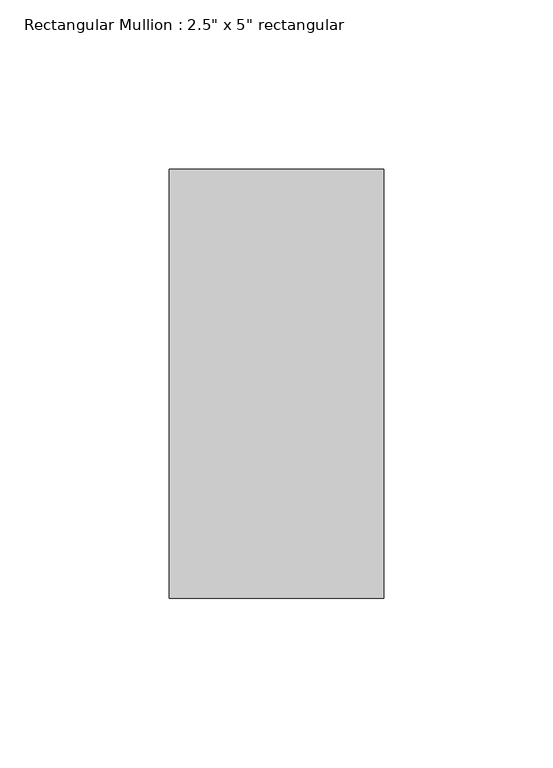
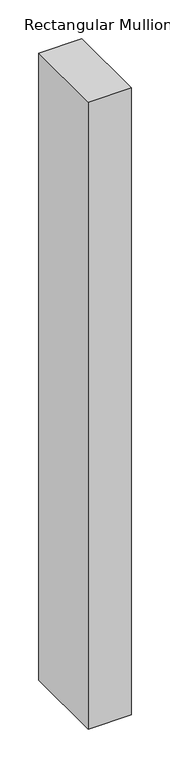
"""IFC4 building model written with IfcOpenShell, lengths in millimetres: member geometry."""

from ifc_helpers import new_model, si_unit, frame, origin, place, context, project, spatial, polyline, outline, extrude, source, transform, mapped, element, save


def member_05cf8435(model_context):
    return source(origin(), model_context, "Body", "SweptSolid", [
        extrude(outline(polyline([(0.0, 63.5), (0.0, -63.5), (-63.5, -63.5), (-63.5, 63.5), (0.0, 63.5)])), frame((0.0, 0.0, -984.3912675), z_axis=(0.0, 0.0, 1.0), x_axis=(1.0, 0.0, 0.0)), (0.0, 0.0, 1.0), 984.3912675),
    ])


if __name__ == "__main__":
    model = new_model("IFC4")
    model_context = context("Model", 3, world=origin())
    ifc_project = project(units=[si_unit("LENGTHUNIT", "METRE", prefix="MILLI")], contexts=[model_context])
    site = spatial("IfcSite", under=ifc_project)
    building = spatial("IfcBuilding", under=site)
    placement = place(None, origin())
    member_shape = member_05cf8435(model_context)
    element("IfcMember", 1, ObjectType="Rectangular Mullion : 2.5\" x 5\" rectangular", at=placement, inside=building, context=model_context, shape_type="MappedRepresentation", body=[
        mapped(member_shape, transform((0.0, 0.0, 0.0), x_axis=(1.0, 0.0, 0.0), y_axis=(0.0, 1.0, 0.0), z_axis=(0.0, 0.0, 1.0))),
    ])
    save(model, "model.ifc")

# Revit data of these elements
# Type "Rectangular Mullion : 2.5\" x 5\" rectangular"
#   built-in parameter 1007304 = 0.416667 (stored number, unit not read)
#   built-in parameter 1007301 = 0.104167 (stored number, unit not read)
#   built-in parameter 1007300 = 0.104167 (stored number, unit not read)
# Element 1 (IfcMember, "Rectangular Mullion : 2.5\" x 5\" rectangular")
#   Materials on its faces: "Aluminum"
# Materials
#   "Aluminum": class "Metal", colour RGB 247 247 247, transparency 0, Description = "Aluminum 6061", Cost = 0
